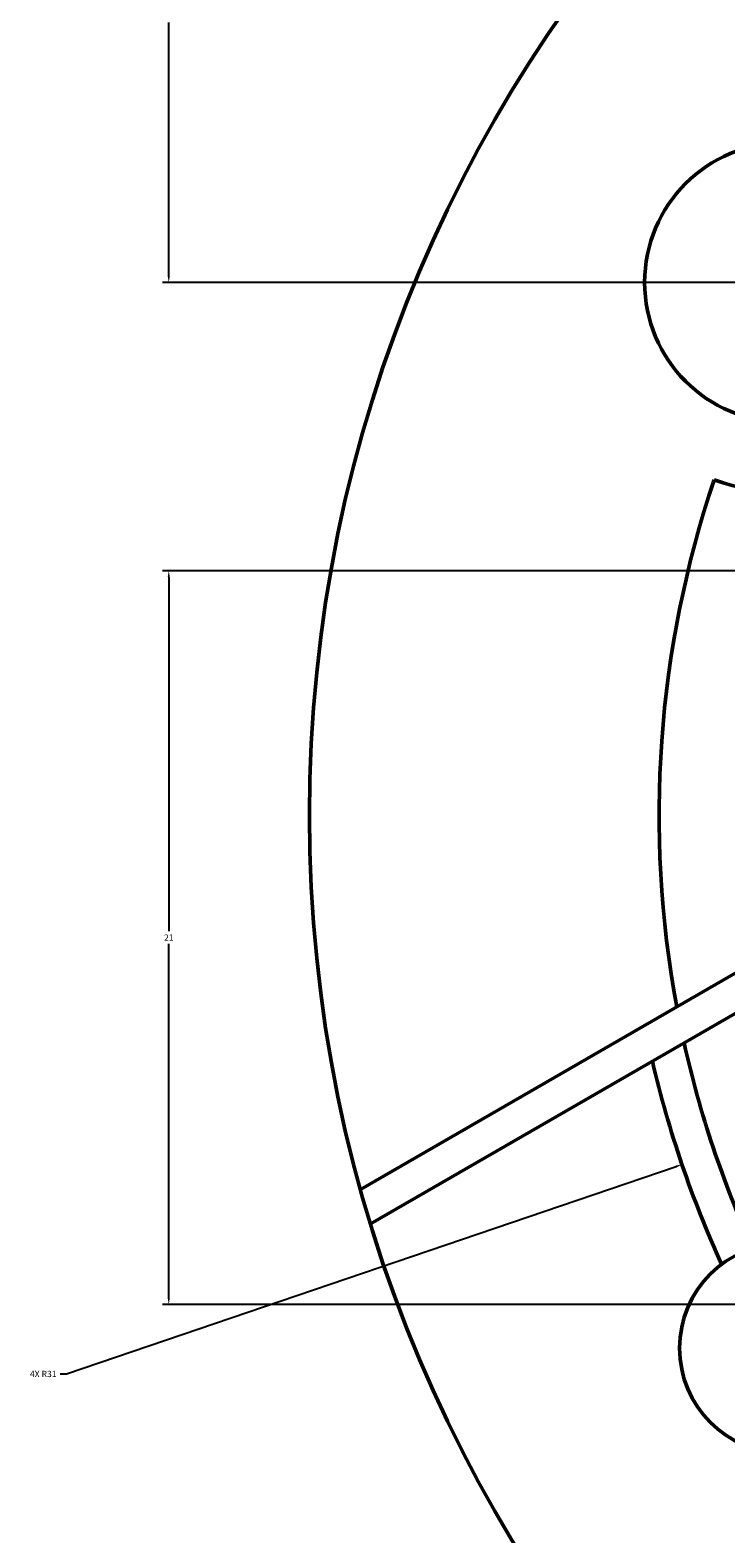
# Model space of a CAD drawing. Units: inches. Extents: x -19.9 to 72.3, y -39.8 to 57.5.
# Tile 2 of 8: x -19.9 to 0, y -7.2 to 35.8. Entities that reach past the tile are written whole.
import ezdxf

# ---------------------------------------------------------------- set-up
doc = ezdxf.new("R2010")
doc.units = ezdxf.units.IN
doc.header["$MEASUREMENT"] = 0
for name, color, linetype, lineweight in [('M-DIMS', 2, 'Continuous', 18), ('M-OUTL', 7, 'Continuous', 50), ('M-OUTL-HOLE', 7, 'Continuous', 50), ('M-OUTL-SLOT', 7, 'Continuous', 50)]:
    doc.layers.add(name, color=color, linetype=linetype, lineweight=lineweight)
doc.styles.get("Standard").update_dxf_attribs({"font": 'arial.ttf'})
doc.dimstyles.get("Standard").update_dxf_attribs({"dimtxt": 0.18, "dimasz": 0.18, "dimexe": 0.18, "dimexo": 0.0625, "dimgap": 0.09, "dimtad": 0, "dimtih": 1, "dimtoh": 1, "dimdec": 4, "dimzin": 0, "dimdsep": 46, "dimtxsty": 'Standard', "dimcen": 0.09, "dimadec": 0, "dimazin": 0, "dimtfac": 1, "dimtdec": 4, "dimtofl": 0, "dimtmove": 0, "dimatfit": 3, "dimfxl": 1, "dimtolj": 1, "dimtzin": 0, "dimarcsym": 0})

# ---------------------------------------------------------------- blocks, each defined once
blk = doc.blocks.new('FLANGE-MOUNT-D8-RELIEVED')
blk.add_circle((0, 0), 4)
for centre, radius, start, end in [((26.414, -15.25), 30, 109.4712, 138.6562), ((0, 0), 6, 250.4286, 49.5714), ((26.414, -15.25), 30, 161.3438, 190.5288)]:
    blk.add_arc(centre, radius, start, end)
blk = doc.blocks.new('FLANGE-HOLE-D6')
blk.add_circle((0, 0), 3)
blk = doc.blocks.new('FLANGE-STRAIGHT-SLOT')
for p, q in [((0, 0), (0, 21.114)), ((1, -0.54), (1, 20.869))]:
    blk.add_line(p, q)
blk = doc.blocks.new('FLANGE-INTERRUPTED-ARC-SLOT')
for radius, start, end in [(30, 192.5424, 204.3948), (31, 193.1227, 204.486), (30, 215.6052, 227.4576), (31, 215.514, 226.8773)]:
    blk.add_arc((26.414, 15.25), radius, start, end)
blk = doc.blocks.new('*D9')
at = {"layer": 'Defpoints', "color": 0, "transparency": 16777216}
for p in [(15.936, 20.341), (-15.966, -0.659), (28.06, -0.659)]:
    blk.add_point(p, dxfattribs=at)
at = {"layer": 'M-DIMS', "color": 0, "lineweight": -2, "transparency": 16777216}
for p, q in [((15.873, 20.341), (-16.146, 20.341)), ((-15.966, 20.161), (-15.966, 10.022)), ((-15.966, -0.479), (-15.966, 9.661)), ((27.997, -0.659), (-16.146, -0.659))]:
    blk.add_line(p, q, dxfattribs=at)
at = {"layer": 'M-DIMS', "color": 0, "transparency": 16777216}
for points in [[(-15.996, 20.161), (-15.936, 20.161), (-15.966, 20.341)], [(-15.996, -0.479), (-15.936, -0.479), (-15.966, -0.659)]]:
    blk.add_solid(points, dxfattribs=at)
at = {"layer": 'M-DIMS', "color": 0, "transparency": 16777216, "insert": (-15.966, 9.841), "char_height": 0.18, "attachment_point": 5}
blk.add_mtext('\\A1;21', dxfattribs=at)
blk = doc.blocks.new('*D10')
at = {"layer": 'Defpoints', "color": 0, "transparency": 16777216}
for p in [(28.06, 43.841), (-15.966, 28.591), (1.646, 28.591)]:
    blk.add_point(p, dxfattribs=at)
at = {"layer": 'M-DIMS', "color": 0, "lineweight": -2, "transparency": 16777216}
for p, q in [((27.997, 43.841), (-16.146, 43.841)), ((-15.966, 43.661), (-15.966, 36.398)), ((-15.966, 28.771), (-15.966, 36.034)), ((1.584, 28.591), (-16.146, 28.591))]:
    blk.add_line(p, q, dxfattribs=at)
at = {"layer": 'M-DIMS', "color": 0, "transparency": 16777216}
for points in [[(-15.996, 43.661), (-15.936, 43.661), (-15.966, 43.841)], [(-15.996, 28.771), (-15.936, 28.771), (-15.966, 28.591)]]:
    blk.add_solid(points, dxfattribs=at)
at = {"layer": 'M-DIMS', "color": 0, "transparency": 16777216, "insert": (-15.966, 36.216), "char_height": 0.18, "attachment_point": 5}
blk.add_mtext('\\A1;15.25', dxfattribs=at)
blk = doc.blocks.new('*D12')
at = {"layer": 'Defpoints', "color": 0, "transparency": 16777216}
for p in [(28.06, 13.341), (-1.285, 3.349)]:
    blk.add_point(p, dxfattribs=at)
at = {"layer": 'M-DIMS', "color": 0, "lineweight": -2, "transparency": 16777216}
for p, q in [((28.06, 13.251), (28.06, 13.431)), ((27.97, 13.341), (28.15, 13.341)), ((-18.893, -2.647), (-1.456, 3.291)), ((-19.073, -2.647), (-18.893, -2.647))]:
    blk.add_line(p, q, dxfattribs=at)
at = {"layer": 'M-DIMS', "color": 0, "transparency": 16777216}
blk.add_solid([(-1.466, 3.319), (-1.446, 3.262), (-1.285, 3.349)], dxfattribs=at)
at = {"layer": 'M-DIMS', "color": 0, "transparency": 16777216, "insert": (-19.557, -2.647), "char_height": 0.18, "attachment_point": 5}
blk.add_mtext('\\A1;4X R31', dxfattribs=at)

msp = doc.modelspace()

# ---------------------------------------------------------------- linework, layer by layer
at = {"layer": 'M-OUTL'}
msp.add_circle((28.06, 13.341), 40, dxfattribs=at)

# ---------------------------------------------------------------- block references
at = {"layer": 'M-OUTL-HOLE'}
for name, p in [('FLANGE-MOUNT-D8-RELIEVED', (1.646, 28.591)), ('FLANGE-HOLE-D6', (1.646, -1.909))]:
    msp.add_blockref(name, p, dxfattribs=at)
at = {"layer": 'M-OUTL-SLOT', "rotation": 119.9999999999999}
msp.add_blockref('FLANGE-STRAIGHT-SLOT', (8.092, 12.205), dxfattribs=at)
at = {"layer": 'M-OUTL-SLOT'}
msp.add_blockref('FLANGE-INTERRUPTED-ARC-SLOT', (1.646, -1.909), dxfattribs=at)
at = {"layer": 'M-OUTL-SLOT', "extrusion": (0, 0, -1), "zscale": -1, "rotation": 239.9999999999999}
msp.add_blockref('FLANGE-STRAIGHT-SLOT', (-17.092, -3.383), dxfattribs=at)

# ---------------------------------------------------------------- dimensions: what is measured, and where the dimension line sits
at = {"layer": 'M-DIMS'}
for base, p1, p2, override, picture, middle in [((-15.966, 28.591), (28.06, 43.841), (1.646, 28.591), {"dimdec": 2, "dimlfac": 1, "dimrnd": 0, "dimzin": 0, "dimdsep": 46, "dimlunit": 2}, '*D10', (-15.966, 36.216)), ((-15.966, -0.659), (15.936, 20.341), (28.06, -0.659), {"dimdec": 0, "dimlfac": 1, "dimrnd": 0, "dimzin": 0, "dimdsep": 46, "dimlunit": 2}, '*D9', (-15.966, 9.841))]:
    dim = msp.add_linear_dim(base=base, p1=p1, p2=p2, angle=90, dimstyle='Standard', override=override, dxfattribs=at)
    dim.commit()
    dim.dimension.update_dxf_attribs({"geometry": picture, "text_midpoint": middle})
dim = msp.add_radius_dim(center=(28.06, 13.341), mpoint=(-1.285, 3.349), text='4X <>', dimstyle='Standard', override={"dimdec": 0, "dimlfac": 1, "dimrnd": 0, "dimzin": 0, "dimdsep": 46, "dimlunit": 2}, dxfattribs=at)
dim.commit()
dim.dimension.update_dxf_attribs({"geometry": '*D12', "text_midpoint": (-19.557, -2.647), "dimtype": 164})

doc.saveas('drawing.dxf')
